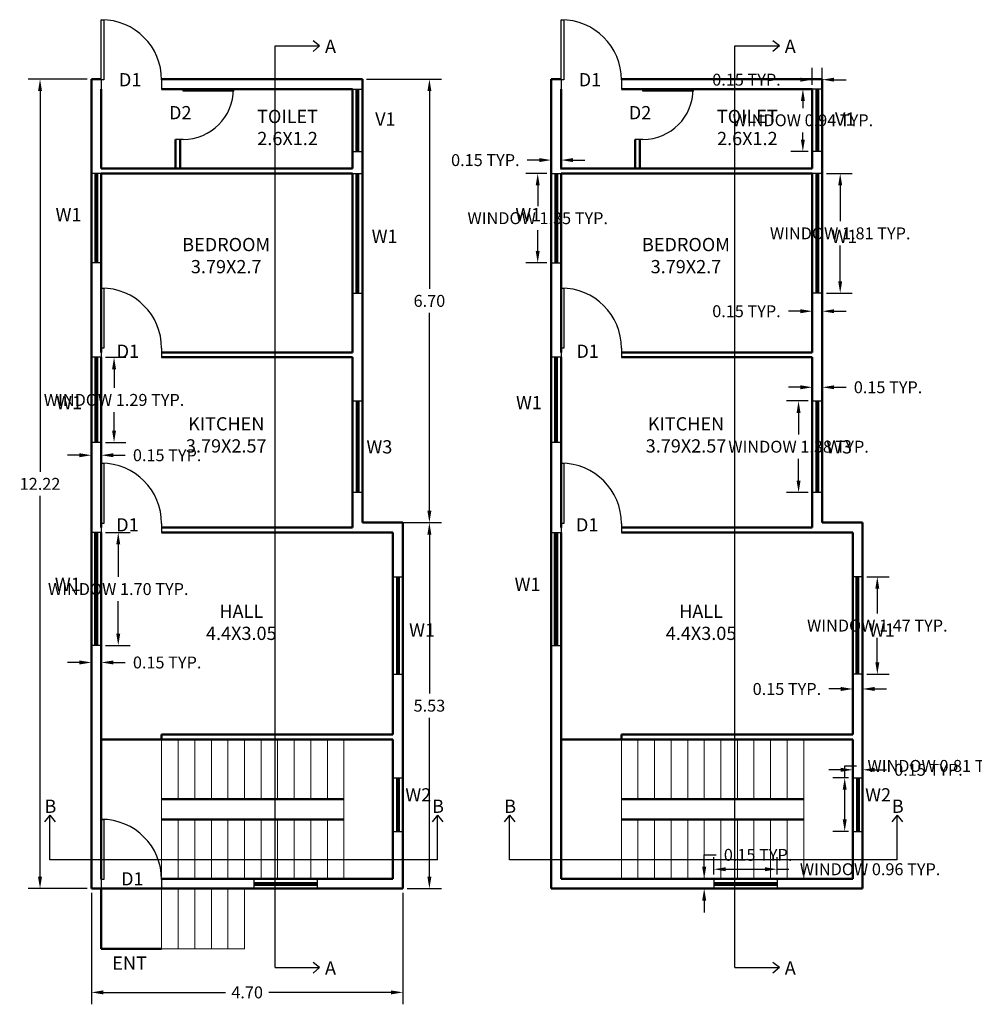
# Model space of a CAD drawing. Units: metres. Extents: x 8.1 to 56.2, y -9.3 to 36.3.
# Tile 2 of 6: x 8.1 to 22.5, y 9.1 to 24. Entities that reach past the tile are written whole.
import ezdxf

# ---------------------------------------------------------------- set-up
doc = ezdxf.new("R2010")
doc.units = ezdxf.units.M
doc.header["$LTSCALE"] = 0.01
doc.header["$MEASUREMENT"] = 0
for name, color, linetype, lineweight in [('A-ANNO-DIMS', 2, 'Continuous', 18), ('A-ANNO-SYMB', 1, 'Continuous', 25), ('A-ANNO-TEXT', 7, 'Continuous', 18), ('A-AREA-IDEN', 3, 'Continuous', 18), ('A-DOOR', 4, 'Continuous', 25), ('A-FLOR-STRS', 8, 'Continuous', 18), ('A-GLAZ', 3, 'Continuous', 25), ('A-WALL', 7, 'Continuous', 50)]:
    doc.layers.add(name, color=color, linetype=linetype, lineweight=lineweight)
doc.styles.get("Standard").update_dxf_attribs({"font": 'arial.ttf'})
doc.dimstyles.get("Standard").update_dxf_attribs({"dimtxt": 0.18, "dimasz": 0.18, "dimexe": 0.18, "dimexo": 0.0625, "dimgap": 0.09, "dimtad": 0, "dimtih": 1, "dimtoh": 1, "dimzin": 0, "dimdsep": 46, "dimtxsty": 'Standard', "dimcen": 0.09, "dimadec": 0, "dimazin": 0, "dimtfac": 1, "dimtofl": 0, "dimtmove": 0, "dimatfit": 3, "dimfxl": 1, "dimtolj": 1, "dimtzin": 0, "dimarcsym": 0})

# ---------------------------------------------------------------- blocks, each defined once
blk = doc.blocks.new('*U2')
for p, q in [((0, 0), (0, -6)), ((40, 0), (40, -6))]:
    blk.add_line(p, q)
blk.add_lwpolyline([(0, 0), (0, 40), (1.75, 40), (1.75, 0)], close=True)
blk.add_arc((0, 0), 40, 0, 90)
blk = doc.blocks.new('*D3')
at = {"layer": 'A-ANNO-DIMS', "color": 0, "lineweight": -2, "transparency": 16777216}
for p, q in [((9.187, 10.82), (9.187, 9.137)), ((13.887, 10.82), (13.887, 9.137)), ((9.367, 9.317), (11.209, 9.317)), ((13.707, 9.317), (11.864, 9.317))]:
    blk.add_line(p, q, dxfattribs=at)
at = {"layer": 'A-ANNO-DIMS', "color": 0, "transparency": 16777216}
for points in [[(9.367, 9.347), (9.367, 9.287), (9.187, 9.317)], [(13.707, 9.347), (13.707, 9.287), (13.887, 9.317)]]:
    blk.add_solid(points, dxfattribs=at)
at = {"layer": 'Defpoints', "color": 0, "transparency": 16777216}
for p in [(9.187, 10.883), (13.887, 10.883), (13.887, 9.317)]:
    blk.add_point(p, dxfattribs=at)
at = {"layer": 'A-ANNO-DIMS', "color": 0, "transparency": 16777216, "insert": (11.537, 9.317), "char_height": 0.18, "attachment_point": 5}
blk.add_mtext('\\A1;4.70', dxfattribs=at)
blk = doc.blocks.new('*D4')
at = {"layer": 'A-ANNO-DIMS', "color": 0, "lineweight": -2, "transparency": 16777216}
for p, q in [((13.339, 23.103), (14.467, 23.103)), ((14.287, 22.923), (14.287, 19.937)), ((14.287, 16.588), (14.287, 19.573)), ((13.339, 16.408), (14.467, 16.408))]:
    blk.add_line(p, q, dxfattribs=at)
at = {"layer": 'A-ANNO-DIMS', "color": 0, "transparency": 16777216}
for points in [[(14.257, 22.923), (14.317, 22.923), (14.287, 23.103)], [(14.257, 16.588), (14.317, 16.588), (14.287, 16.408)]]:
    blk.add_solid(points, dxfattribs=at)
at = {"layer": 'Defpoints', "color": 0, "transparency": 16777216}
for p in [(13.277, 23.103), (13.277, 16.408), (14.287, 16.408)]:
    blk.add_point(p, dxfattribs=at)
at = {"layer": 'A-ANNO-DIMS', "color": 0, "transparency": 16777216, "insert": (14.287, 19.755), "char_height": 0.18, "attachment_point": 5}
blk.add_mtext('\\A1;6.70', dxfattribs=at)
blk = doc.blocks.new('*D5')
at = {"layer": 'A-ANNO-DIMS', "color": 0, "lineweight": -2, "transparency": 16777216}
for p, q in [((13.949, 16.408), (14.467, 16.408)), ((14.287, 16.228), (14.287, 13.827)), ((14.287, 11.063), (14.287, 13.463)), ((13.949, 10.883), (14.467, 10.883))]:
    blk.add_line(p, q, dxfattribs=at)
at = {"layer": 'A-ANNO-DIMS', "color": 0, "transparency": 16777216}
for points in [[(14.257, 16.228), (14.317, 16.228), (14.287, 16.408)], [(14.257, 11.063), (14.317, 11.063), (14.287, 10.883)]]:
    blk.add_solid(points, dxfattribs=at)
at = {"layer": 'Defpoints', "color": 0, "transparency": 16777216}
for p in [(13.887, 16.408), (13.887, 10.883), (14.287, 10.883)]:
    blk.add_point(p, dxfattribs=at)
at = {"layer": 'A-ANNO-DIMS', "color": 0, "transparency": 16777216, "insert": (14.287, 13.645), "char_height": 0.18, "attachment_point": 5}
blk.add_mtext('\\A1;5.53', dxfattribs=at)
blk = doc.blocks.new('*D6')
at = {"layer": 'A-ANNO-DIMS', "color": 0, "lineweight": -2, "transparency": 16777216}
for p, q in [((9.124, 23.103), (8.232, 23.103)), ((8.412, 22.923), (8.412, 17.173)), ((8.412, 11.063), (8.412, 16.812)), ((9.124, 10.883), (8.232, 10.883))]:
    blk.add_line(p, q, dxfattribs=at)
at = {"layer": 'A-ANNO-DIMS', "color": 0, "transparency": 16777216}
for points in [[(8.382, 22.923), (8.442, 22.923), (8.412, 23.103)], [(8.382, 11.063), (8.442, 11.063), (8.412, 10.883)]]:
    blk.add_solid(points, dxfattribs=at)
at = {"layer": 'Defpoints', "color": 0, "transparency": 16777216}
for p in [(8.412, 23.103), (9.187, 23.103), (9.187, 10.883)]:
    blk.add_point(p, dxfattribs=at)
at = {"layer": 'A-ANNO-DIMS', "color": 0, "transparency": 16777216, "insert": (8.412, 16.993), "char_height": 0.18, "attachment_point": 5}
blk.add_mtext('\\A1;12.22', dxfattribs=at)
blk = doc.blocks.new('WIN-PLAN-810')
for p, q in [((0, 0.808), (0.15, 0.808)), ((0.055, 0.808), (0.055, 0)), ((0.075, 0.808), (0.075, 0)), ((0.095, 0.808), (0.095, 0)), ((0, 0), (0.15, 0))]:
    blk.add_line(p, q)
blk = doc.blocks.new('WIN-PLAN-1470')
for p, q in [((0, 1.472), (0.15, 1.472)), ((0.055, 1.472), (0.055, 0)), ((0.075, 1.472), (0.075, 0)), ((0.095, 1.472), (0.095, 0)), ((0, 0), (0.15, 0))]:
    blk.add_line(p, q)
blk = doc.blocks.new('WIN-PLAN-1380')
for p, q in [((0, 1.381), (0.15, 1.381)), ((0.055, 1.381), (0.055, 0)), ((0.075, 1.381), (0.075, 0)), ((0.095, 1.381), (0.095, 0)), ((0.15, 0), (0, 0))]:
    blk.add_line(p, q)
blk = doc.blocks.new('WIN-PLAN-1810')
for p, q in [((0, 1.808), (0.15, 1.808)), ((0.055, 0), (0.055, 1.808)), ((0.075, 0), (0.075, 1.808)), ((0.095, 0), (0.095, 1.808)), ((0, 0), (0.15, 0))]:
    blk.add_line(p, q)
blk = doc.blocks.new('WIN-PLAN-940')
for p, q in [((0, 0.943), (0.15, 0.943)), ((0.055, 0), (0.055, 0.943)), ((0.075, 0), (0.075, 0.943)), ((0.095, 0), (0.095, 0.943)), ((0, 0), (0.15, 0))]:
    blk.add_line(p, q)
blk = doc.blocks.new('WIN-PLAN-1350')
for p, q in [((0.15, 1.35), (0, 1.35)), ((0.055, 0), (0.055, 1.35)), ((0.075, 0), (0.075, 1.35)), ((0.095, 0), (0.095, 1.35)), ((0.15, 0), (0, 0))]:
    blk.add_line(p, q)
blk = doc.blocks.new('WIN-PLAN-1290')
for p, q in [((0.15, 1.285), (0, 1.285)), ((0.055, 0), (0.055, 1.285)), ((0.075, 0), (0.075, 1.285)), ((0.095, 0), (0.095, 1.285)), ((0.15, 0), (0, 0))]:
    blk.add_line(p, q)
blk = doc.blocks.new('WIN-PLAN-1700')
for p, q in [((0.15, 1.705), (0, 1.705)), ((0.055, 0), (0.055, 1.705)), ((0.075, 0), (0.075, 1.705)), ((0.095, 0), (0.095, 1.705)), ((0.15, 0), (0, 0))]:
    blk.add_line(p, q)
blk = doc.blocks.new('WIN-PLAN-950')
for p, q in [((0, 0.15), (0, 0)), ((0.956, 0.15), (0.956, 0)), ((0, 0.095), (0.956, 0.095)), ((0, 0.075), (0.956, 0.075)), ((0, 0.055), (0.956, 0.055))]:
    blk.add_line(p, q)
blk = doc.blocks.new('*D47')
at = {"layer": 'A-ANNO-DIMS', "color": 0, "lineweight": -2, "ltscale": 0.01, "transparency": 16777216}
for p, q in [((20.553, 12.556), (20.553, 12.736)), ((20.553, 12.736), (20.733, 12.736)), ((20.611, 12.556), (20.373, 12.556)), ((20.553, 11.928), (20.553, 12.376)), ((20.611, 11.748), (20.373, 11.748))]:
    blk.add_line(p, q, dxfattribs=at)
at = {"layer": 'A-ANNO-DIMS', "color": 0, "ltscale": 0.01, "transparency": 16777216}
for points in [[(20.523, 12.376), (20.583, 12.376), (20.553, 12.556)], [(20.523, 11.928), (20.583, 11.928), (20.553, 11.748)]]:
    blk.add_solid(points, dxfattribs=at)
at = {"layer": 'Defpoints', "color": 0, "ltscale": 0.01, "transparency": 16777216}
for p in [(20.553, 12.556), (20.674, 12.556), (20.674, 11.748)]:
    blk.add_point(p, dxfattribs=at)
at = {"layer": 'A-ANNO-DIMS', "color": 0, "ltscale": 0.01, "transparency": 16777216, "insert": (21.956, 12.736), "char_height": 0.18, "attachment_point": 5}
blk.add_mtext('\\A1;WINDOW 0.81 TYP.', dxfattribs=at)
blk = doc.blocks.new('*D48')
at = {"layer": 'A-ANNO-DIMS', "color": 0, "lineweight": -2, "ltscale": 0.01, "transparency": 16777216}
for p, q in [((20.674, 12.618), (20.674, 12.857)), ((20.824, 12.618), (20.824, 12.857)), ((20.494, 12.677), (20.314, 12.677)), ((21.004, 12.677), (21.184, 12.677))]:
    blk.add_line(p, q, dxfattribs=at)
at = {"layer": 'A-ANNO-DIMS', "color": 0, "ltscale": 0.01, "transparency": 16777216}
for points in [[(20.494, 12.707), (20.494, 12.647), (20.674, 12.677)], [(21.004, 12.707), (21.004, 12.647), (20.824, 12.677)]]:
    blk.add_solid(points, dxfattribs=at)
at = {"layer": 'Defpoints', "color": 0, "ltscale": 0.01, "transparency": 16777216}
for p in [(20.824, 12.677), (20.674, 12.556), (20.824, 12.556)]:
    blk.add_point(p, dxfattribs=at)
at = {"layer": 'A-ANNO-DIMS', "color": 0, "ltscale": 0.01, "transparency": 16777216, "insert": (21.817, 12.677), "char_height": 0.18, "attachment_point": 5}
blk.add_mtext('\\A1;0.15 TYP.', dxfattribs=at)
blk = doc.blocks.new('*D49')
at = {"layer": 'A-ANNO-DIMS', "color": 0, "lineweight": -2, "ltscale": 0.01, "transparency": 16777216}
for p, q in [((20.886, 15.59), (21.225, 15.59)), ((21.045, 15.41), (21.045, 15.037)), ((21.045, 14.298), (21.045, 14.671)), ((20.886, 14.118), (21.225, 14.118))]:
    blk.add_line(p, q, dxfattribs=at)
at = {"layer": 'A-ANNO-DIMS', "color": 0, "ltscale": 0.01, "transparency": 16777216}
for points in [[(21.015, 15.41), (21.075, 15.41), (21.045, 15.59)], [(21.015, 14.298), (21.075, 14.298), (21.045, 14.118)]]:
    blk.add_solid(points, dxfattribs=at)
at = {"layer": 'Defpoints', "color": 0, "ltscale": 0.01, "transparency": 16777216}
for p in [(20.824, 15.59), (20.824, 14.118), (21.045, 14.118)]:
    blk.add_point(p, dxfattribs=at)
at = {"layer": 'A-ANNO-DIMS', "color": 0, "ltscale": 0.01, "transparency": 16777216, "insert": (21.045, 14.854), "char_height": 0.18, "attachment_point": 5}
blk.add_mtext('\\A1;WINDOW 1.47 TYP.', dxfattribs=at)
blk = doc.blocks.new('*D50')
at = {"layer": 'A-ANNO-DIMS', "color": 0, "lineweight": -2, "ltscale": 0.01, "transparency": 16777216}
for p, q in [((20.674, 14.055), (20.674, 13.717)), ((20.824, 14.055), (20.824, 13.717)), ((20.494, 13.897), (20.314, 13.897)), ((21.004, 13.897), (21.184, 13.897))]:
    blk.add_line(p, q, dxfattribs=at)
at = {"layer": 'A-ANNO-DIMS', "color": 0, "ltscale": 0.01, "transparency": 16777216}
for points in [[(20.494, 13.927), (20.494, 13.867), (20.674, 13.897)], [(21.004, 13.927), (21.004, 13.867), (20.824, 13.897)]]:
    blk.add_solid(points, dxfattribs=at)
at = {"layer": 'Defpoints', "color": 0, "ltscale": 0.01, "transparency": 16777216}
for p in [(20.674, 14.118), (20.824, 14.118), (20.674, 13.897)]:
    blk.add_point(p, dxfattribs=at)
at = {"layer": 'A-ANNO-DIMS', "color": 0, "ltscale": 0.01, "transparency": 16777216, "insert": (19.681, 13.897), "char_height": 0.18, "attachment_point": 5}
blk.add_mtext('\\A1;0.15 TYP.', dxfattribs=at)
blk = doc.blocks.new('*D51')
at = {"layer": 'A-ANNO-DIMS', "color": 0, "lineweight": -2, "ltscale": 0.01, "transparency": 16777216}
for p, q in [((20.001, 18.244), (19.677, 18.244)), ((19.857, 18.064), (19.857, 17.737)), ((19.857, 17.043), (19.857, 17.37)), ((20.001, 16.863), (19.677, 16.863))]:
    blk.add_line(p, q, dxfattribs=at)
at = {"layer": 'A-ANNO-DIMS', "color": 0, "ltscale": 0.01, "transparency": 16777216}
for points in [[(19.827, 18.064), (19.887, 18.064), (19.857, 18.244)], [(19.827, 17.043), (19.887, 17.043), (19.857, 16.863)]]:
    blk.add_solid(points, dxfattribs=at)
at = {"layer": 'Defpoints', "color": 0, "ltscale": 0.01, "transparency": 16777216}
for p in [(19.857, 18.244), (20.064, 18.244), (20.064, 16.863)]:
    blk.add_point(p, dxfattribs=at)
at = {"layer": 'A-ANNO-DIMS', "color": 0, "ltscale": 0.01, "transparency": 16777216, "insert": (19.857, 17.554), "char_height": 0.18, "attachment_point": 5}
blk.add_mtext('\\A1;WINDOW 1.38 TYP.', dxfattribs=at)
blk = doc.blocks.new('*D52')
at = {"layer": 'A-ANNO-DIMS', "color": 0, "lineweight": -2, "ltscale": 0.01, "transparency": 16777216}
for p, q in [((20.064, 18.307), (20.064, 18.631)), ((20.214, 18.307), (20.214, 18.631)), ((19.884, 18.451), (19.704, 18.451)), ((20.394, 18.451), (20.574, 18.451))]:
    blk.add_line(p, q, dxfattribs=at)
at = {"layer": 'A-ANNO-DIMS', "color": 0, "ltscale": 0.01, "transparency": 16777216}
for points in [[(19.884, 18.481), (19.884, 18.421), (20.064, 18.451)], [(20.394, 18.481), (20.394, 18.421), (20.214, 18.451)]]:
    blk.add_solid(points, dxfattribs=at)
at = {"layer": 'Defpoints', "color": 0, "ltscale": 0.01, "transparency": 16777216}
for p in [(20.214, 18.451), (20.064, 18.244), (20.214, 18.244)]:
    blk.add_point(p, dxfattribs=at)
at = {"layer": 'A-ANNO-DIMS', "color": 0, "ltscale": 0.01, "transparency": 16777216, "insert": (21.207, 18.451), "char_height": 0.18, "attachment_point": 5}
blk.add_mtext('\\A1;0.15 TYP.', dxfattribs=at)
blk = doc.blocks.new('*D53')
at = {"layer": 'A-ANNO-DIMS', "color": 0, "lineweight": -2, "ltscale": 0.01, "transparency": 16777216}
for p, q in [((20.276, 21.678), (20.665, 21.678)), ((20.485, 21.498), (20.485, 20.957)), ((20.485, 20.05), (20.485, 20.591)), ((20.276, 19.87), (20.665, 19.87))]:
    blk.add_line(p, q, dxfattribs=at)
at = {"layer": 'A-ANNO-DIMS', "color": 0, "ltscale": 0.01, "transparency": 16777216}
for points in [[(20.455, 21.498), (20.515, 21.498), (20.485, 21.678)], [(20.455, 20.05), (20.515, 20.05), (20.485, 19.87)]]:
    blk.add_solid(points, dxfattribs=at)
at = {"layer": 'Defpoints', "color": 0, "ltscale": 0.01, "transparency": 16777216}
for p in [(20.214, 21.678), (20.214, 19.87), (20.485, 19.87)]:
    blk.add_point(p, dxfattribs=at)
at = {"layer": 'A-ANNO-DIMS', "color": 0, "ltscale": 0.01, "transparency": 16777216, "insert": (20.485, 20.774), "char_height": 0.18, "attachment_point": 5}
blk.add_mtext('\\A1;WINDOW 1.81 TYP.', dxfattribs=at)
blk = doc.blocks.new('*D54')
at = {"layer": 'A-ANNO-DIMS', "color": 0, "lineweight": -2, "ltscale": 0.01, "transparency": 16777216}
for p, q in [((20.064, 19.808), (20.064, 19.419)), ((20.214, 19.808), (20.214, 19.419)), ((19.884, 19.599), (19.704, 19.599)), ((20.394, 19.599), (20.574, 19.599))]:
    blk.add_line(p, q, dxfattribs=at)
at = {"layer": 'A-ANNO-DIMS', "color": 0, "ltscale": 0.01, "transparency": 16777216}
for points in [[(19.884, 19.629), (19.884, 19.569), (20.064, 19.599)], [(20.394, 19.629), (20.394, 19.569), (20.214, 19.599)]]:
    blk.add_solid(points, dxfattribs=at)
at = {"layer": 'Defpoints', "color": 0, "ltscale": 0.01, "transparency": 16777216}
for p in [(20.064, 19.87), (20.214, 19.87), (20.064, 19.599)]:
    blk.add_point(p, dxfattribs=at)
at = {"layer": 'A-ANNO-DIMS', "color": 0, "ltscale": 0.01, "transparency": 16777216, "insert": (19.071, 19.599), "char_height": 0.18, "attachment_point": 5}
blk.add_mtext('\\A1;0.15 TYP.', dxfattribs=at)
blk = doc.blocks.new('*D55')
at = {"layer": 'A-ANNO-DIMS', "color": 0, "lineweight": -2, "ltscale": 0.01, "transparency": 16777216}
for p, q in [((20.001, 22.953), (19.742, 22.953)), ((19.922, 22.773), (19.922, 22.665)), ((19.922, 22.19), (19.922, 22.298)), ((20.001, 22.01), (19.742, 22.01))]:
    blk.add_line(p, q, dxfattribs=at)
at = {"layer": 'A-ANNO-DIMS', "color": 0, "ltscale": 0.01, "transparency": 16777216}
for points in [[(19.892, 22.773), (19.952, 22.773), (19.922, 22.953)], [(19.892, 22.19), (19.952, 22.19), (19.922, 22.01)]]:
    blk.add_solid(points, dxfattribs=at)
at = {"layer": 'Defpoints', "color": 0, "ltscale": 0.01, "transparency": 16777216}
for p in [(20.064, 22.953), (19.922, 22.01), (20.064, 22.01)]:
    blk.add_point(p, dxfattribs=at)
at = {"layer": 'A-ANNO-DIMS', "color": 0, "ltscale": 0.01, "transparency": 16777216, "insert": (19.922, 22.481), "char_height": 0.18, "attachment_point": 5}
blk.add_mtext('\\A1;WINDOW 0.94 TYP.', dxfattribs=at)
blk = doc.blocks.new('*D56')
at = {"layer": 'A-ANNO-DIMS', "color": 0, "lineweight": -2, "ltscale": 0.01, "transparency": 16777216}
for p, q in [((20.064, 23.015), (20.064, 23.274)), ((20.214, 23.015), (20.214, 23.274)), ((19.884, 23.094), (19.704, 23.094)), ((20.394, 23.094), (20.574, 23.094))]:
    blk.add_line(p, q, dxfattribs=at)
at = {"layer": 'A-ANNO-DIMS', "color": 0, "ltscale": 0.01, "transparency": 16777216}
for points in [[(19.884, 23.124), (19.884, 23.064), (20.064, 23.094)], [(20.394, 23.124), (20.394, 23.064), (20.214, 23.094)]]:
    blk.add_solid(points, dxfattribs=at)
at = {"layer": 'Defpoints', "color": 0, "ltscale": 0.01, "transparency": 16777216}
for p in [(20.064, 23.094), (20.064, 22.953), (20.214, 22.953)]:
    blk.add_point(p, dxfattribs=at)
at = {"layer": 'A-ANNO-DIMS', "color": 0, "ltscale": 0.01, "transparency": 16777216, "insert": (19.071, 23.094), "char_height": 0.18, "attachment_point": 5}
blk.add_mtext('\\A1;0.15 TYP.', dxfattribs=at)
blk = doc.blocks.new('*D57')
at = {"layer": 'A-ANNO-DIMS', "color": 0, "lineweight": -2, "ltscale": 0.01, "transparency": 16777216}
for p, q in [((16.061, 21.678), (15.741, 21.678)), ((15.921, 21.498), (15.921, 21.186)), ((15.921, 20.508), (15.921, 20.82)), ((16.061, 20.328), (15.741, 20.328))]:
    blk.add_line(p, q, dxfattribs=at)
at = {"layer": 'A-ANNO-DIMS', "color": 0, "ltscale": 0.01, "transparency": 16777216}
for points in [[(15.891, 21.498), (15.951, 21.498), (15.921, 21.678)], [(15.891, 20.508), (15.951, 20.508), (15.921, 20.328)]]:
    blk.add_solid(points, dxfattribs=at)
at = {"layer": 'Defpoints', "color": 0, "ltscale": 0.01, "transparency": 16777216}
for p in [(16.124, 21.678), (15.921, 20.328), (16.124, 20.328)]:
    blk.add_point(p, dxfattribs=at)
at = {"layer": 'A-ANNO-DIMS', "color": 0, "ltscale": 0.01, "transparency": 16777216, "insert": (15.921, 21.003), "char_height": 0.18, "attachment_point": 5}
blk.add_mtext('\\A1;WINDOW 1.35 TYP.', dxfattribs=at)
blk = doc.blocks.new('*D58')
at = {"layer": 'A-ANNO-DIMS', "color": 0, "lineweight": -2, "ltscale": 0.01, "transparency": 16777216}
for p, q in [((16.124, 21.74), (16.124, 22.06)), ((16.274, 21.74), (16.274, 22.06)), ((15.944, 21.88), (15.764, 21.88)), ((16.454, 21.88), (16.634, 21.88))]:
    blk.add_line(p, q, dxfattribs=at)
at = {"layer": 'A-ANNO-DIMS', "color": 0, "ltscale": 0.01, "transparency": 16777216}
for points in [[(15.944, 21.91), (15.944, 21.85), (16.124, 21.88)], [(16.454, 21.91), (16.454, 21.85), (16.274, 21.88)]]:
    blk.add_solid(points, dxfattribs=at)
at = {"layer": 'Defpoints', "color": 0, "ltscale": 0.01, "transparency": 16777216}
for p in [(16.124, 21.88), (16.124, 21.678), (16.274, 21.678)]:
    blk.add_point(p, dxfattribs=at)
at = {"layer": 'A-ANNO-DIMS', "color": 0, "ltscale": 0.01, "transparency": 16777216, "insert": (15.131, 21.88), "char_height": 0.18, "attachment_point": 5}
blk.add_mtext('\\A1;0.15 TYP.', dxfattribs=at)
blk = doc.blocks.new('*D59')
at = {"layer": 'A-ANNO-DIMS', "color": 0, "lineweight": -2, "ltscale": 0.01, "transparency": 16777216}
for p, q in [((9.399, 18.903), (9.709, 18.903)), ((9.529, 18.723), (9.529, 18.443)), ((9.529, 17.798), (9.529, 18.077)), ((9.399, 17.618), (9.709, 17.618))]:
    blk.add_line(p, q, dxfattribs=at)
at = {"layer": 'A-ANNO-DIMS', "color": 0, "ltscale": 0.01, "transparency": 16777216}
for points in [[(9.499, 18.723), (9.559, 18.723), (9.529, 18.903)], [(9.499, 17.798), (9.559, 17.798), (9.529, 17.618)]]:
    blk.add_solid(points, dxfattribs=at)
at = {"layer": 'Defpoints', "color": 0, "ltscale": 0.01, "transparency": 16777216}
for p in [(9.337, 18.903), (9.529, 18.903), (9.337, 17.618)]:
    blk.add_point(p, dxfattribs=at)
at = {"layer": 'A-ANNO-DIMS', "color": 0, "ltscale": 0.01, "transparency": 16777216, "insert": (9.529, 18.26), "char_height": 0.18, "attachment_point": 5}
blk.add_mtext('\\A1;WINDOW 1.29 TYP.', dxfattribs=at)
blk = doc.blocks.new('*D60')
at = {"layer": 'A-ANNO-DIMS', "color": 0, "lineweight": -2, "ltscale": 0.01, "transparency": 16777216}
for p, q in [((9.187, 17.555), (9.187, 17.245)), ((9.337, 17.555), (9.337, 17.245)), ((9.007, 17.425), (8.827, 17.425)), ((9.517, 17.425), (9.697, 17.425))]:
    blk.add_line(p, q, dxfattribs=at)
at = {"layer": 'A-ANNO-DIMS', "color": 0, "ltscale": 0.01, "transparency": 16777216}
for points in [[(9.007, 17.455), (9.007, 17.395), (9.187, 17.425)], [(9.517, 17.455), (9.517, 17.395), (9.337, 17.425)]]:
    blk.add_solid(points, dxfattribs=at)
at = {"layer": 'Defpoints', "color": 0, "ltscale": 0.01, "transparency": 16777216}
for p in [(9.187, 17.618), (9.337, 17.618), (9.337, 17.425)]:
    blk.add_point(p, dxfattribs=at)
at = {"layer": 'A-ANNO-DIMS', "color": 0, "ltscale": 0.01, "transparency": 16777216, "insert": (10.33, 17.425), "char_height": 0.18, "attachment_point": 5}
blk.add_mtext('\\A1;0.15 TYP.', dxfattribs=at)
blk = doc.blocks.new('*D61')
at = {"layer": 'A-ANNO-DIMS', "color": 0, "lineweight": -2, "ltscale": 0.01, "transparency": 16777216}
for p, q in [((9.399, 16.258), (9.772, 16.258)), ((9.592, 16.078), (9.592, 15.589)), ((9.592, 14.733), (9.592, 15.222)), ((9.399, 14.553), (9.772, 14.553))]:
    blk.add_line(p, q, dxfattribs=at)
at = {"layer": 'A-ANNO-DIMS', "color": 0, "ltscale": 0.01, "transparency": 16777216}
for points in [[(9.562, 16.078), (9.622, 16.078), (9.592, 16.258)], [(9.562, 14.733), (9.622, 14.733), (9.592, 14.553)]]:
    blk.add_solid(points, dxfattribs=at)
at = {"layer": 'Defpoints', "color": 0, "ltscale": 0.01, "transparency": 16777216}
for p in [(9.337, 16.258), (9.592, 16.258), (9.337, 14.553)]:
    blk.add_point(p, dxfattribs=at)
at = {"layer": 'A-ANNO-DIMS', "color": 0, "ltscale": 0.01, "transparency": 16777216, "insert": (9.592, 15.405), "char_height": 0.18, "attachment_point": 5}
blk.add_mtext('\\A1;WINDOW 1.70 TYP.', dxfattribs=at)
blk = doc.blocks.new('*D62')
at = {"layer": 'A-ANNO-DIMS', "color": 0, "lineweight": -2, "ltscale": 0.01, "transparency": 16777216}
for p, q in [((9.187, 14.491), (9.187, 14.117)), ((9.337, 14.491), (9.337, 14.117)), ((9.007, 14.297), (8.827, 14.297)), ((9.517, 14.297), (9.697, 14.297))]:
    blk.add_line(p, q, dxfattribs=at)
at = {"layer": 'A-ANNO-DIMS', "color": 0, "ltscale": 0.01, "transparency": 16777216}
for points in [[(9.007, 14.327), (9.007, 14.267), (9.187, 14.297)], [(9.517, 14.327), (9.517, 14.267), (9.337, 14.297)]]:
    blk.add_solid(points, dxfattribs=at)
at = {"layer": 'Defpoints', "color": 0, "ltscale": 0.01, "transparency": 16777216}
for p in [(9.187, 14.553), (9.337, 14.553), (9.337, 14.297)]:
    blk.add_point(p, dxfattribs=at)
at = {"layer": 'A-ANNO-DIMS', "color": 0, "ltscale": 0.01, "transparency": 16777216, "insert": (10.33, 14.297), "char_height": 0.18, "attachment_point": 5}
blk.add_mtext('\\A1;0.15 TYP.', dxfattribs=at)
blk = doc.blocks.new('*D63')
at = {"layer": 'A-ANNO-DIMS', "color": 0, "lineweight": -2, "ltscale": 0.01, "transparency": 16777216}
for p, q in [((18.577, 11.095), (18.577, 11.356)), ((19.532, 11.095), (19.532, 11.356)), ((18.757, 11.176), (19.352, 11.176)), ((19.532, 11.176), (19.712, 11.176))]:
    blk.add_line(p, q, dxfattribs=at)
at = {"layer": 'A-ANNO-DIMS', "color": 0, "ltscale": 0.01, "transparency": 16777216}
for points in [[(18.757, 11.206), (18.757, 11.146), (18.577, 11.176)], [(19.352, 11.206), (19.352, 11.146), (19.532, 11.176)]]:
    blk.add_solid(points, dxfattribs=at)
at = {"layer": 'Defpoints', "color": 0, "ltscale": 0.01, "transparency": 16777216}
for p in [(19.532, 11.176), (18.577, 11.033), (19.532, 11.033)]:
    blk.add_point(p, dxfattribs=at)
at = {"layer": 'A-ANNO-DIMS', "color": 0, "ltscale": 0.01, "transparency": 16777216, "insert": (20.936, 11.176), "char_height": 0.18, "attachment_point": 5}
blk.add_mtext('\\A1;WINDOW 0.96 TYP.', dxfattribs=at)
blk = doc.blocks.new('*D64')
at = {"layer": 'A-ANNO-DIMS', "color": 0, "lineweight": -2, "ltscale": 0.01, "transparency": 16777216}
for p, q in [((18.433, 11.213), (18.433, 11.393)), ((18.433, 11.393), (18.613, 11.393)), ((18.514, 11.033), (18.253, 11.033)), ((18.514, 10.883), (18.253, 10.883)), ((18.433, 10.703), (18.433, 10.523))]:
    blk.add_line(p, q, dxfattribs=at)
at = {"layer": 'A-ANNO-DIMS', "color": 0, "ltscale": 0.01, "transparency": 16777216}
for points in [[(18.403, 11.213), (18.463, 11.213), (18.433, 11.033)], [(18.403, 10.703), (18.463, 10.703), (18.433, 10.883)]]:
    blk.add_solid(points, dxfattribs=at)
at = {"layer": 'Defpoints', "color": 0, "ltscale": 0.01, "transparency": 16777216}
for p in [(18.433, 11.033), (18.577, 11.033), (18.577, 10.883)]:
    blk.add_point(p, dxfattribs=at)
at = {"layer": 'A-ANNO-DIMS', "color": 0, "ltscale": 0.01, "transparency": 16777216, "insert": (19.246, 11.393), "char_height": 0.18, "attachment_point": 5}
blk.add_mtext('\\A1;0.15 TYP.', dxfattribs=at)

msp = doc.modelspace()

# ---------------------------------------------------------------- linework, layer by layer
at = {"layer": 'A-ANNO-SYMB'}
for p, q in [((12.63, 23.603), (12.533, 23.681)), ((19.567, 23.603), (19.47, 23.681)), ((11.959, 9.691), (11.959, 23.603)), ((11.959, 23.603), (12.63, 23.603)), ((12.63, 23.603), (12.533, 23.52)), ((18.896, 9.691), (18.896, 23.603)), ((18.896, 23.603), (19.567, 23.603)), ((19.567, 23.603), (19.47, 23.52)), ((8.558, 11.991), (8.48, 11.894)), ((8.558, 11.32), (8.558, 11.991)), ((8.558, 11.991), (8.641, 11.894)), ((14.407, 11.991), (14.329, 11.894)), ((14.407, 11.32), (14.407, 11.991)), ((14.407, 11.991), (14.489, 11.894)), ((15.495, 11.991), (15.417, 11.894)), ((15.495, 11.32), (15.495, 11.991)), ((15.495, 11.991), (15.578, 11.894)), ((21.344, 11.991), (21.266, 11.894)), ((21.344, 11.32), (21.344, 11.991)), ((21.344, 11.991), (21.427, 11.894)), ((14.407, 11.32), (8.558, 11.32)), ((21.344, 11.32), (15.495, 11.32)), ((11.959, 9.691), (12.63, 9.691)), ((12.63, 9.691), (12.533, 9.769)), ((12.63, 9.691), (12.533, 9.608)), ((18.896, 9.691), (19.567, 9.691)), ((19.567, 9.691), (19.47, 9.769)), ((19.567, 9.691), (19.47, 9.608))]:
    msp.add_line(p, q, dxfattribs=at)
at = {"layer": 'A-FLOR-STRS'}
for p, q in [((10.247, 13.133), (10.247, 12.236)), ((10.497, 13.133), (10.497, 12.236)), ((10.747, 13.133), (10.747, 12.236)), ((10.997, 13.133), (10.997, 12.236)), ((11.247, 13.133), (11.247, 12.236)), ((11.497, 13.133), (11.497, 12.236)), ((11.747, 13.133), (11.747, 12.236)), ((11.997, 13.133), (11.997, 12.236)), ((12.247, 13.133), (12.247, 12.236)), ((12.497, 13.133), (12.497, 12.236)), ((12.747, 13.133), (12.747, 12.236)), ((12.997, 13.133), (12.997, 12.236)), ((17.184, 13.133), (17.184, 12.236)), ((17.434, 13.133), (17.434, 12.236)), ((17.684, 13.133), (17.684, 12.236)), ((17.934, 13.133), (17.934, 12.236)), ((18.184, 13.133), (18.184, 12.236)), ((18.434, 13.133), (18.434, 12.236)), ((18.684, 13.133), (18.684, 12.236)), ((18.934, 13.133), (18.934, 12.236)), ((19.184, 13.133), (19.184, 12.236)), ((19.434, 13.133), (19.434, 12.236)), ((19.684, 13.133), (19.684, 12.236)), ((19.934, 13.133), (19.934, 12.236)), ((10.247, 12.236), (10.247, 11.929)), ((12.997, 11.929), (12.997, 12.236)), ((17.184, 12.236), (17.184, 11.929)), ((19.934, 11.929), (19.934, 12.236)), ((10.247, 11.019), (10.247, 11.929)), ((10.497, 11.033), (10.497, 11.929)), ((10.747, 11.033), (10.747, 11.929)), ((10.997, 11.033), (10.997, 11.929)), ((11.247, 11.033), (11.247, 11.929)), ((11.497, 11.033), (11.497, 11.929)), ((11.747, 11.033), (11.747, 11.929)), ((11.997, 11.033), (11.997, 11.929)), ((12.247, 11.033), (12.247, 11.929)), ((12.497, 11.033), (12.497, 11.929)), ((12.747, 11.033), (12.747, 11.929)), ((12.997, 11.033), (12.997, 11.929)), ((17.184, 11.033), (17.184, 11.929)), ((17.434, 11.033), (17.434, 11.929)), ((17.684, 11.033), (17.684, 11.929)), ((17.934, 11.033), (17.934, 11.929)), ((18.184, 11.033), (18.184, 11.929)), ((18.434, 11.033), (18.434, 11.929)), ((18.684, 11.033), (18.684, 11.929)), ((18.934, 11.033), (18.934, 11.929)), ((19.184, 11.033), (19.184, 11.929)), ((19.434, 11.033), (19.434, 11.929)), ((19.684, 11.033), (19.684, 11.929)), ((19.934, 11.033), (19.934, 11.929)), ((10.247, 10.883), (10.247, 9.973)), ((10.497, 10.883), (10.497, 9.973)), ((10.747, 10.883), (10.747, 9.973)), ((10.997, 10.883), (10.997, 9.973)), ((11.247, 10.883), (11.247, 9.973)), ((11.497, 10.883), (11.497, 9.973)), ((11.497, 9.973), (10.247, 9.973))]:
    msp.add_line(p, q, dxfattribs=at)
at = {"layer": 'A-WALL'}
for p, q in [((9.187, 23.103), (9.337, 23.103)), ((9.187, 23.103), (9.187, 10.883)), ((10.246, 23.103), (13.277, 23.103)), ((13.277, 23.103), (13.277, 16.408)), ((16.124, 23.103), (16.274, 23.103)), ((16.124, 23.103), (16.124, 10.883)), ((17.184, 23.103), (20.214, 23.103)), ((20.214, 23.103), (20.214, 16.408)), ((9.337, 22.953), (9.337, 21.753)), ((10.247, 22.953), (13.127, 22.953)), ((13.127, 22.953), (13.127, 21.753)), ((16.274, 22.953), (16.274, 21.753)), ((17.184, 22.953), (20.064, 22.953)), ((20.064, 22.953), (20.064, 21.753)), ((10.457, 22.193), (10.457, 21.753)), ((10.527, 22.193), (10.527, 21.753)), ((17.394, 22.193), (17.394, 21.753)), ((17.464, 22.193), (17.464, 21.753)), ((9.337, 21.753), (13.127, 21.753)), ((16.274, 21.753), (20.064, 21.753)), ((9.337, 21.678), (13.127, 21.678)), ((9.337, 21.678), (9.337, 18.978)), ((13.127, 21.678), (13.127, 18.978)), ((16.274, 21.678), (20.064, 21.678)), ((16.274, 21.678), (16.274, 18.978)), ((20.064, 21.678), (20.064, 18.978)), ((9.337, 18.903), (9.337, 16.333)), ((10.247, 18.978), (13.127, 18.978)), ((10.247, 18.903), (13.127, 18.903)), ((13.127, 18.903), (13.127, 16.333)), ((16.274, 18.903), (16.274, 16.333)), ((17.184, 18.978), (20.064, 18.978)), ((17.184, 18.903), (20.064, 18.903)), ((20.064, 18.903), (20.064, 16.333)), ((13.887, 16.408), (13.277, 16.408)), ((13.887, 16.408), (13.887, 10.883)), ((20.824, 16.408), (20.214, 16.408)), ((20.824, 16.408), (20.824, 10.883)), ((9.242, 14.553), (9.242, 16.258)), ((9.337, 16.258), (9.337, 13.208)), ((10.247, 16.333), (13.127, 16.333)), ((10.247, 16.258), (13.277, 16.258)), ((13.737, 16.258), (13.277, 16.258)), ((13.737, 16.258), (13.737, 13.208)), ((16.179, 14.553), (16.179, 16.258)), ((16.274, 16.258), (16.274, 13.208)), ((17.184, 16.333), (20.064, 16.333)), ((17.184, 16.258), (20.214, 16.258)), ((20.674, 16.258), (20.214, 16.258)), ((20.674, 16.258), (20.674, 13.208)), ((9.337, 13.133), (9.337, 13.208)), ((9.337, 13.133), (9.337, 11.033)), ((10.247, 13.133), (9.337, 13.133)), ((10.247, 13.208), (13.737, 13.208)), ((10.247, 13.133), (10.247, 13.208)), ((10.247, 13.133), (13.737, 13.133)), ((13.737, 13.133), (13.737, 11.033)), ((16.274, 13.208), (16.274, 13.133)), ((16.274, 13.133), (16.274, 11.033)), ((17.184, 13.133), (16.274, 13.133)), ((17.184, 13.208), (20.674, 13.208)), ((17.184, 13.208), (17.184, 13.133)), ((17.184, 13.133), (20.674, 13.133)), ((20.674, 13.133), (20.674, 11.033)), ((12.997, 12.236), (10.247, 12.236)), ((19.934, 12.236), (17.184, 12.236)), ((10.247, 11.929), (12.997, 11.929)), ((17.184, 11.929), (19.934, 11.929)), ((10.246, 11.033), (13.737, 11.033)), ((17.184, 11.033), (16.274, 11.033)), ((17.184, 11.033), (20.674, 11.033)), ((9.187, 10.883), (9.337, 10.883)), ((10.247, 10.883), (9.337, 10.883)), ((9.337, 10.883), (9.337, 9.973)), ((10.247, 10.883), (13.887, 10.883)), ((16.124, 10.883), (16.274, 10.883)), ((17.184, 10.883), (16.274, 10.883)), ((17.184, 10.883), (20.824, 10.883)), ((10.247, 9.973), (9.337, 9.973))]:
    msp.add_line(p, q, dxfattribs=at)

# ---------------------------------------------------------------- block references
at = {"layer": 'A-DOOR', "xscale": 0.02275, "yscale": 0.02275, "zscale": 0.02275}
for p in [(9.337, 23.089), (16.274, 23.089), (9.337, 19.039), (16.274, 19.039), (9.337, 16.394), (16.274, 16.394), (9.337, 11.019)]:
    msp.add_blockref('*U2', p, dxfattribs=at)
at = {"layer": 'A-DOOR', "xscale": 0.019, "yscale": 0.019, "zscale": 0.019, "rotation": 270}
for p in [(10.571, 22.953), (17.508, 22.953)]:
    msp.add_blockref('*U2', p, dxfattribs=at)
at = {"layer": 'A-GLAZ'}
for name, p in [('WIN-PLAN-940', (13.127, 22.01)), ('WIN-PLAN-1350', (9.187, 20.328)), ('WIN-PLAN-1810', (13.127, 19.87)), ('WIN-PLAN-1290', (9.187, 17.618)), ('WIN-PLAN-1290', (16.124, 17.618)), ('WIN-PLAN-1380', (13.127, 16.863)), ('WIN-PLAN-1380', (20.064, 16.863)), ('WIN-PLAN-1700', (9.187, 14.553)), ('WIN-PLAN-1470', (13.737, 14.118)), ('WIN-PLAN-810', (13.737, 11.748)), ('WIN-PLAN-810', (20.674, 11.748)), ('WIN-PLAN-950', (11.639, 10.883)), ('WIN-PLAN-950', (18.576, 10.883))]:
    msp.add_blockref(name, p, dxfattribs=at)
at = {"layer": 'A-GLAZ', "rotation": 180}
for name, p in [('WIN-PLAN-940', (20.213, 22.953)), ('WIN-PLAN-1350', (16.273, 21.678)), ('WIN-PLAN-1810', (20.213, 21.678)), ('WIN-PLAN-1700', (16.273, 16.258)), ('WIN-PLAN-1470', (20.823, 15.59))]:
    msp.add_blockref(name, p, dxfattribs=at)

# ---------------------------------------------------------------- texts
at = {"layer": 'A-ANNO-SYMB', "char_height": 0.2, "attachment_point": 1}
for s, insert in [('\\pxqc;A', (12.533, 23.697)), ('\\pxqc;A', (19.47, 23.697)), ('\\pxqc;B', (8.307, 12.227)), ('\\pxqc;B', (14.155, 12.227)), ('\\pxqc;B', (15.244, 12.227)), ('\\pxqc;B', (21.092, 12.227)), ('\\pxqc;A', (12.533, 9.785)), ('\\pxqc;A', (19.47, 9.785))]:
    msp.add_mtext_dynamic_manual_height_columns(s, width=0.52297, gutter_width=1, heights=[0], dxfattribs=dict(at, insert=insert))
at = {"layer": 'A-ANNO-TEXT', "char_height": 0.2, "attachment_point": 1}
for s, width, insert in [('\\pxqc;D1', 0.84791, (9.348, 23.193)), ('\\pxqc;D1', 0.84791, (16.285, 23.193)), ('\\pxqc;D2', 0.84791, (10.104, 22.696)), ('\\pxqc;V1', 0.54589, (13.35, 22.599)), ('\\pxqc;D2', 0.84791, (17.041, 22.696)), ('\\pxqc;V1', 0.54589, (20.288, 22.599)), ('\\pxqc;W1', 0.54589, (8.569, 21.157)), ('\\pxqc;W1', 0.54589, (15.506, 21.157)), ('\\pxqc;W1', 0.54589, (13.338, 20.83)), ('\\pxqc;W1', 0.54589, (20.275, 20.83)), ('\\pxqc;D1', 0.84791, (9.314, 19.095)), ('\\pxqc;D1', 0.84791, (16.251, 19.095)), ('\\pxqc;W1', 0.54589, (8.578, 18.32)), ('\\pxqc;W1', 0.54589, (15.516, 18.32)), ('\\pxqc;W3', 0.54589, (13.259, 17.652)), ('\\pxqc;W3', 0.54589, (20.196, 17.652)), ('\\pxqc;D1', 0.84791, (9.307, 16.475)), ('\\pxqc;D1', 0.84791, (16.244, 16.475)), ('\\pxqc;W1', 0.54589, (8.558, 15.577)), ('\\pxqc;W1', 0.54589, (15.495, 15.577)), ('\\pxqc;W1', 0.54589, (13.903, 14.886)), ('\\pxqc;W1', 0.54589, (20.84, 14.886)), ('\\pxqc;W2', 0.84791, (13.695, 12.399)), ('\\pxqc;W2', 0.84791, (20.633, 12.399)), ('\\pxqc;D1', 0.84791, (9.381, 11.131)), ('\\pxqc;ENT', 0.84791, (9.339, 9.86))]:
    msp.add_mtext_dynamic_manual_height_columns(s, width=width, gutter_width=1, heights=[0], dxfattribs=dict(at, insert=insert))
at = {"layer": 'A-AREA-IDEN', "char_height": 0.2, "attachment_point": 1}
for s, insert in [('\\pxqc;TOILET\\P2.6X1.2', (11.338, 22.639)), ('\\pxqc;TOILET\\P2.6X1.2', (18.275, 22.639)), ('\\pxqc;BEDROOM\\P3.79X2.7', (10.412, 20.705)), ('\\pxqc;BEDROOM\\P3.79X2.7', (17.349, 20.705)), ('\\pxqc;KITCHEN\\P3.79X2.57', (10.413, 17.999)), ('\\pxqc;KITCHEN\\P3.79X2.57', (17.35, 17.999)), ('\\pxqc;HALL\\P4.4X3.05', (10.64, 15.17)), ('\\pxqc;HALL\\P4.4X3.05', (17.577, 15.17))]:
    msp.add_mtext_dynamic_manual_height_columns(s, width=1.61769, gutter_width=1, heights=[0], dxfattribs=dict(at, insert=insert))

# ---------------------------------------------------------------- dimensions: what is measured, and where the dimension line sits
at = {"layer": 'A-ANNO-DIMS', "ltscale": 0.01}
for base, p1, p2, angle, text, picture, middle in [((20.064, 23.094), (20.214, 22.953), (20.064, 22.953), 180, '<> TYP.', '*D56', (19.071, 23.094)), ((19.922, 22.01), (20.064, 22.953), (20.064, 22.01), 270, 'WINDOW <> TYP.', '*D55', (19.922, 22.481)), ((16.124, 21.88), (16.274, 21.678), (16.124, 21.678), 180, '<> TYP.', '*D58', (15.131, 21.88)), ((15.921, 20.328), (16.124, 21.678), (16.124, 20.328), 270, 'WINDOW <> TYP.', '*D57', (15.921, 21.003)), ((20.485, 19.87), (20.214, 21.678), (20.214, 19.87), 270, 'WINDOW <> TYP.', '*D53', (20.485, 20.774)), ((20.064, 19.599), (20.214, 19.87), (20.064, 19.87), 180, '<> TYP.', '*D54', (19.071, 19.599)), ((9.529342223, 18.902777426), (9.336592223, 17.617777426), (9.336592223, 18.902777426), 90, 'WINDOW <> TYP.', '*D59', (9.529342223, 18.260277426)), ((19.857, 18.244), (20.064, 16.863), (20.064, 18.244), 90, 'WINDOW <> TYP.', '*D51', (19.857, 17.554)), ((9.5923, 16.2578), (9.3366, 14.553), (9.3366, 16.2578), 90, 'WINDOW <> TYP.', '*D61', (9.5923, 15.4054)), ((21.045, 14.118), (20.824, 15.59), (20.824, 14.118), 270, 'WINDOW <> TYP.', '*D49', (21.045, 14.854)), ((20.674, 13.897), (20.824, 14.118), (20.674, 14.118), 180, '<> TYP.', '*D50', (19.681, 13.897)), ((20.553, 12.556), (20.674, 11.748), (20.674, 12.556), 90, 'WINDOW <> TYP.', '*D47', (21.956, 12.736)), ((18.433, 11.033), (18.577, 10.883), (18.577, 11.033), 90, '<> TYP.', '*D64', (19.246, 11.393))]:
    dim = msp.add_linear_dim(base=base, p1=p1, p2=p2, angle=angle, text=text, dimstyle='Standard', override={"dimdec": 2, "dimrnd": 0, "dimzin": 0, "dimlunit": 2}, dxfattribs=at)
    dim.commit()
    dim.dimension.update_dxf_attribs({"geometry": picture, "text_midpoint": middle})
at = {"layer": 'A-ANNO-DIMS'}
for base, p1, p2, picture, middle in [((8.412, 23.103), (9.187, 10.883), (9.187, 23.103), '*D6', (8.412, 16.993)), ((14.28654058, 16.407777426), (13.276592223, 23.102777426), (13.276592223, 16.407777426), '*D4', (14.28654058, 19.755277426)), ((14.28654058, 10.882777426), (13.886592223, 16.407777426), (13.886592223, 10.882777426), '*D5', (14.28654058, 13.645277426))]:
    dim = msp.add_linear_dim(base=base, p1=p1, p2=p2, angle=90, dimstyle='Standard', override={"dimclrd": 0, "dimclre": 0, "dimclrt": 0}, dxfattribs=at)
    dim.commit()
    dim.dimension.update_dxf_attribs({"geometry": picture, "text_midpoint": middle})
at = {"layer": 'A-ANNO-DIMS', "ltscale": 0.01}
for base, p1, p2, text, picture, middle in [((20.214, 18.451), (20.064, 18.244), (20.214, 18.244), '<> TYP.', '*D52', (21.207, 18.451)), ((9.337, 17.425), (9.187, 17.618), (9.337, 17.618), '<> TYP.', '*D60', (10.33, 17.425)), ((9.337, 14.297), (9.187, 14.553), (9.337, 14.553), '<> TYP.', '*D62', (10.33, 14.297)), ((20.824, 12.677), (20.674, 12.556), (20.824, 12.556), '<> TYP.', '*D48', (21.817, 12.677)), ((19.5324, 11.1761), (18.5766, 11.0328), (19.5324, 11.0328), 'WINDOW <> TYP.', '*D63', (20.9356, 11.1761))]:
    dim = msp.add_linear_dim(base=base, p1=p1, p2=p2, text=text, dimstyle='Standard', override={"dimdec": 2, "dimrnd": 0, "dimzin": 0, "dimlunit": 2}, dxfattribs=at)
    dim.commit()
    dim.dimension.update_dxf_attribs({"geometry": picture, "text_midpoint": middle})
at = {"layer": 'A-ANNO-DIMS'}
dim = msp.add_linear_dim(base=(13.887, 9.317), p1=(9.187, 10.883), p2=(13.887, 10.883), dimstyle='Standard', override={"dimclrd": 0, "dimclre": 0, "dimclrt": 0}, dxfattribs=at)
dim.commit()
dim.dimension.update_dxf_attribs({"geometry": '*D3', "text_midpoint": (11.537, 9.317)})

doc.saveas('drawing.dxf')
